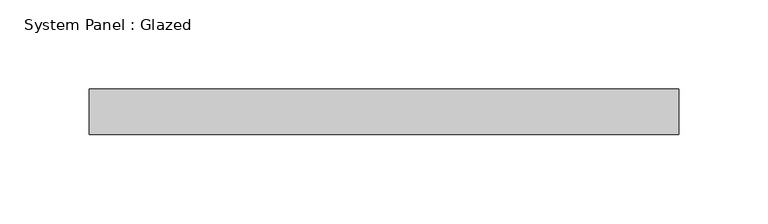
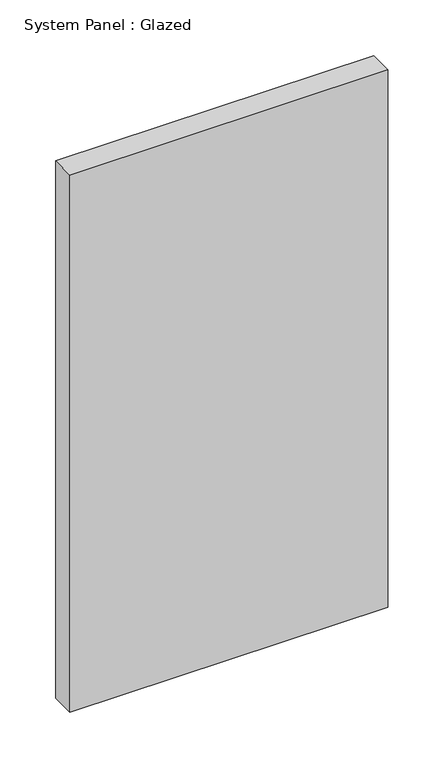
"""IFC4 building model written with IfcOpenShell, lengths in millimetres: plate geometry, System Panel : Glazed."""

from ifc_helpers import new_model, si_unit, origin, origin_with_axes, place, context, project, spatial, polyline, outline, extrude, source, transform, mapped, element, save


def system_panel_glazed_8b3a0672(model_context):
    return source(origin(), model_context, "Body", "SweptSolid", [
        extrude(outline(polyline([(165.1, 19.05), (-165.1, 19.05), (-165.1, 44.45), (165.1, 44.45), (165.1, 19.05)])), origin_with_axes(), (0.0, 0.0, 1.0), 589.5522733),
    ])


if __name__ == "__main__":
    model = new_model("IFC4")
    model_context = context("Model", 3, world=origin())
    ifc_project = project(units=[si_unit("LENGTHUNIT", "METRE", prefix="MILLI")], contexts=[model_context])
    site = spatial("IfcSite", under=ifc_project)
    building = spatial("IfcBuilding", under=site)
    placement = place(None, origin())
    system_panel_glazed_shape = system_panel_glazed_8b3a0672(model_context)
    element("IfcPlate", 1, ObjectType="System Panel : Glazed", at=placement, inside=building, context=model_context, shape_type="MappedRepresentation", body=[
        mapped(system_panel_glazed_shape, transform((0.0, 0.0, 0.0), x_axis=(1.0, 0.0, 0.0), y_axis=(0.0, 1.0, 0.0), z_axis=(0.0, 0.0, 1.0))),
    ])
    save(model, "model.ifc")

# Revit data of these elements
# Type "System Panel : Glazed"
#   Construction Type Id = "GSP4R"
#   Analytic Construction = "1/8 in Pilkington single glazing"
#   Visual Light Transmittance = 0.9
#   Solar Heat Gain Coefficient = 0.86
#   Heat Transfer Coefficient (U) = 1.18115 BTU/(h·ft²·°F)
#   Define Thermal Properties by = 1
# Element 1 (IfcPlate, "System Panel : Glazed")
#   Materials on its faces: "Glass"
# Materials
#   "Glass": class "Glass", colour RGB 0 128 192, transparency 0.75, Description = "Soda Lime Glass", Cost = 0
